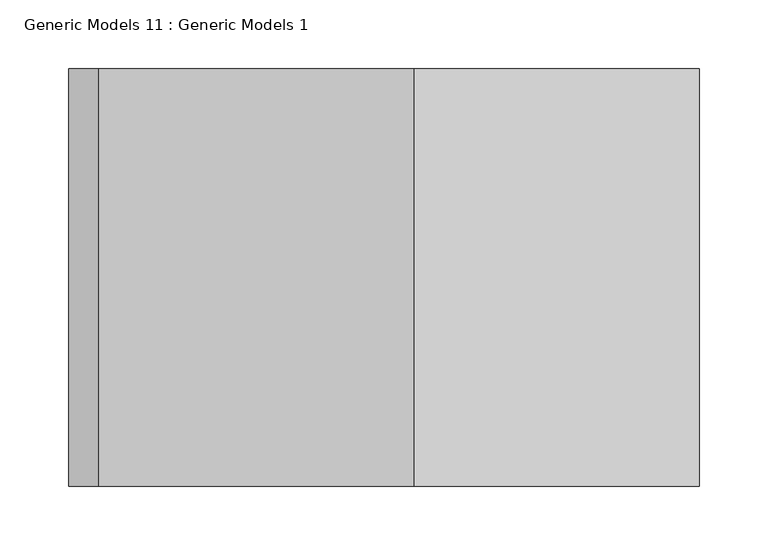
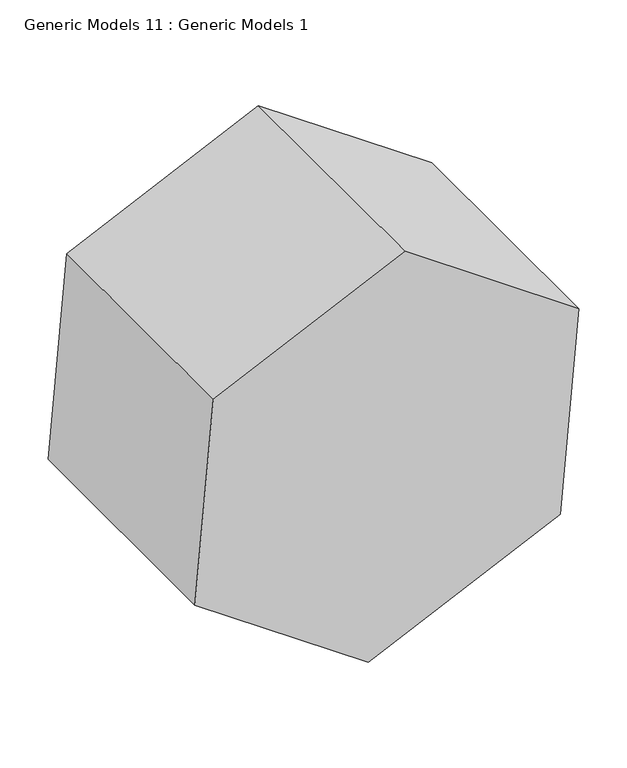
"""IFC4 building model written with IfcOpenShell, lengths in millimetres: proxy geometry, Generic Models 11 : Generic Models 1."""

from ifc_helpers import new_model, si_unit, frame, origin, place, context, project, spatial, polyline, outline, extrude, source, transform, mapped, element, save


def generic_models_11_generic_models_1_35dd710a(model_context):
    return source(origin(), model_context, "Body", "SweptSolid", [
        extrude(outline(polyline([(833.1013393, 2638.0920945), (978.7897542, 2430.0274753), (871.4447157, 2199.8252974), (618.4112624, 2177.6877387), (472.7228475, 2385.752358), (580.067886, 2615.9545359), (833.1013393, 2638.0920945)])), frame((0.0, -10720.3372434, 0.0), z_axis=(0.0, 1.0, 0.0), x_axis=(0.0, 0.0, 1.0)), (0.0, 0.0, 1.0), 304.8),
    ])


if __name__ == "__main__":
    model = new_model("IFC4")
    model_context = context("Model", 3, world=origin())
    ifc_project = project(units=[si_unit("LENGTHUNIT", "METRE", prefix="MILLI")], contexts=[model_context])
    site = spatial("IfcSite", under=ifc_project)
    building = spatial("IfcBuilding", under=site)
    placement = place(None, origin())
    generic_models_11_generic_models_1_shape = generic_models_11_generic_models_1_35dd710a(model_context)
    element("IfcBuildingElementProxy", 1, Name="Generic Models 11 : Generic Models 1", ObjectType="Generic Models 11 : Generic Models 1", at=placement, inside=building, context=model_context, shape_type="MappedRepresentation", body=[
        mapped(generic_models_11_generic_models_1_shape, transform((0.0, 0.0, 0.0), x_axis=(1.0, 0.0, 0.0), y_axis=(0.0, 1.0, 0.0), z_axis=(0.0, 0.0, 1.0))),
    ])
    save(model, "model.ifc")
